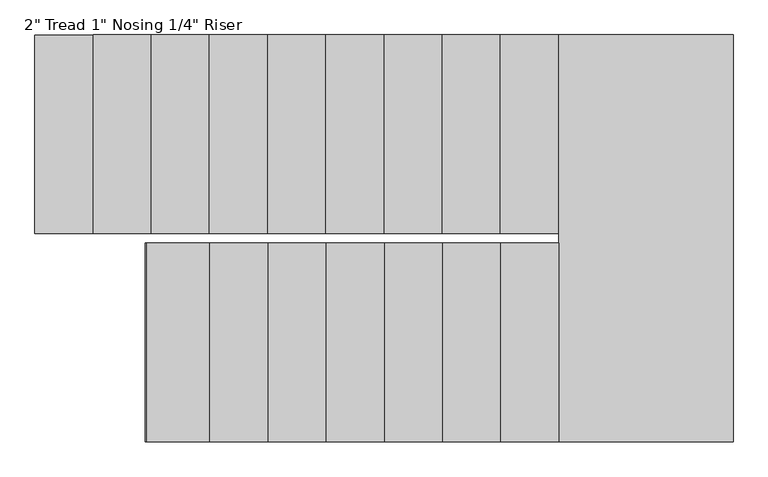
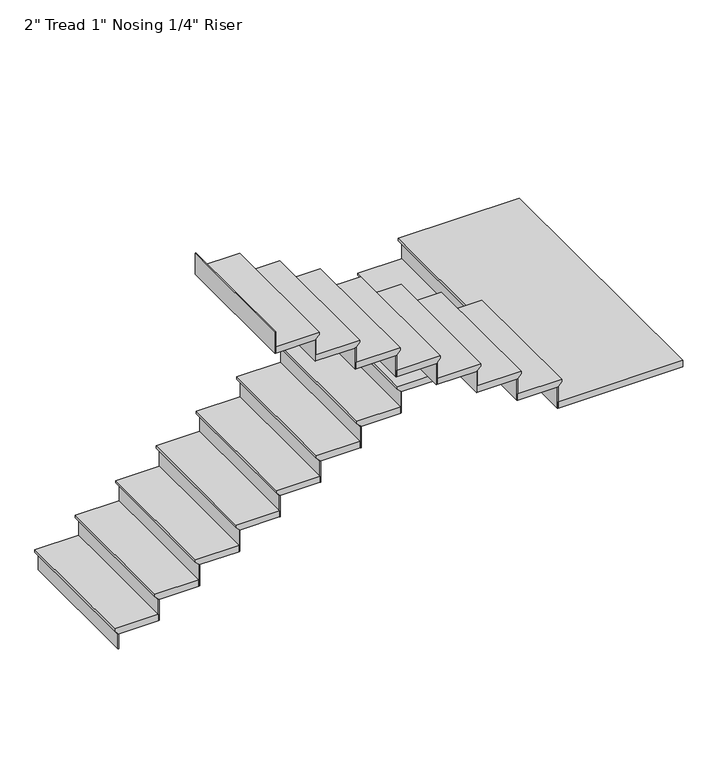
"""IFC4 building model written with IfcOpenShell, lengths in millimetres: stair flight geometry."""

from ifc_helpers import new_model, si_unit, origin, place, context, project, spatial, faceted_brep, source, transform, mapped, element, save


def stair_flight_e0aa27d8(model_context):
    return source(origin(), model_context, "Body", "Brep", [
        faceted_brep([(1775.9671209, 2655.5223211, 455.0833333), (1775.9671209, 2655.5223211, 474.1333333), (1775.9671209, 3696.9223211, 474.1333333), (1775.9671209, 3696.9223211, 455.0833333), (1801.3671209, 2655.5223211, 429.6833333), (1801.3671209, 3696.9223211, 429.6833333), (2106.1671209, 2655.5223211, 474.1333333), (2106.1671209, 3696.9223211, 474.1333333), (1801.3671209, 3696.9223211, 423.3333333), (2106.1671209, 3696.9223211, 423.3333333), (2106.1671209, 2655.5223211, 423.3333333), (1801.3671209, 2655.5223211, 423.3333333)], [[[0, 1, 2, 3]], [[4, 0, 3, 5]], [[2, 1, 6, 7]], [[8, 9, 10, 11]], [[2, 7, 9, 8, 5, 3]], [[8, 11, 4, 5]], [[6, 1, 0, 4, 11, 10]], [[7, 6, 10, 9]]]),
        faceted_brep([(1801.3671209, 2655.5223211, 423.3333333), (1801.3671209, 2655.5223211, 304.8), (1807.7171209, 2655.5223211, 304.8), (1807.7171209, 2655.5223211, 423.3333333), (1801.3671209, 3696.9223211, 423.3333333), (1807.7171209, 3696.9223211, 423.3333333), (1807.7171209, 3696.9223211, 304.8), (1801.3671209, 3696.9223211, 304.8)], [[[0, 1, 2, 3]], [[4, 5, 6, 7]], [[1, 0, 4, 7]], [[2, 1, 7, 6]], [[3, 2, 6, 5]], [[0, 3, 5, 4]]]),
        faceted_brep([(2106.1671209, 2655.5223211, 592.6666667), (2106.1671209, 2655.5223211, 423.3333333), (2112.5171209, 2655.5223211, 423.3333333), (2112.5171209, 2655.5223211, 592.6666667), (2106.1671209, 3696.9223211, 592.6666667), (2112.5171209, 3696.9223211, 592.6666667), (2112.5171209, 3696.9223211, 423.3333333), (2106.1671209, 3696.9223211, 423.3333333)], [[[0, 1, 2, 3]], [[4, 5, 6, 7]], [[1, 0, 4, 7]], [[2, 1, 7, 6]], [[3, 2, 6, 5]], [[0, 3, 5, 4]]]),
        faceted_brep([(2080.7671209, 3696.9223211, 643.4666667), (2080.7671209, 2655.5223211, 643.4666667), (2410.9671209, 2655.5223211, 643.4666667), (2410.9671209, 3696.9223211, 643.4666667), (2106.1671209, 3696.9223211, 592.6666667), (2410.9671209, 3696.9223211, 592.6666667), (2410.9671209, 2655.5223211, 592.6666667), (2106.1671209, 2655.5223211, 592.6666667), (2106.1671209, 3696.9223211, 599.0166667), (2080.7671209, 3696.9223211, 624.4166667), (2106.1671209, 2655.5223211, 599.0166667), (2080.7671209, 2655.5223211, 624.4166667)], [[[0, 1, 2, 3]], [[4, 5, 6, 7]], [[0, 3, 5, 4, 8, 9]], [[4, 7, 10, 8]], [[2, 1, 11, 10, 7, 6]], [[3, 2, 6, 5]], [[11, 1, 0, 9]], [[10, 11, 9, 8]]]),
        faceted_brep([(2410.9671209, 2655.5223211, 762.0), (2410.9671209, 2655.5223211, 592.6666667), (2417.3171209, 2655.5223211, 592.6666667), (2417.3171209, 2655.5223211, 762.0), (2410.9671209, 3696.9223211, 762.0), (2417.3171209, 3696.9223211, 762.0), (2417.3171209, 3696.9223211, 592.6666667), (2410.9671209, 3696.9223211, 592.6666667)], [[[0, 1, 2, 3]], [[4, 5, 6, 7]], [[1, 0, 4, 7]], [[2, 1, 7, 6]], [[3, 2, 6, 5]], [[0, 3, 5, 4]]]),
        faceted_brep([(2385.5671209, 3696.9223211, 812.8), (2385.5671209, 2655.5223211, 812.8), (2715.7671209, 2655.5223211, 812.8), (2715.7671209, 3696.9223211, 812.8), (2410.9671209, 3696.9223211, 762.0), (2715.7671209, 3696.9223211, 762.0), (2715.7671209, 2655.5223211, 762.0), (2410.9671209, 2655.5223211, 762.0), (2410.9671209, 3696.9223211, 768.35), (2385.5671209, 3696.9223211, 793.75), (2410.9671209, 2655.5223211, 768.35), (2385.5671209, 2655.5223211, 793.75)], [[[0, 1, 2, 3]], [[4, 5, 6, 7]], [[0, 3, 5, 4, 8, 9]], [[4, 7, 10, 8]], [[2, 1, 11, 10, 7, 6]], [[3, 2, 6, 5]], [[11, 1, 0, 9]], [[10, 11, 9, 8]]]),
        faceted_brep([(2715.7671209, 2655.5223211, 931.3333333), (2715.7671209, 2655.5223211, 762.0), (2722.1171209, 2655.5223211, 762.0), (2722.1171209, 2655.5223211, 931.3333333), (2715.7671209, 3696.9223211, 931.3333333), (2722.1171209, 3696.9223211, 931.3333333), (2722.1171209, 3696.9223211, 762.0), (2715.7671209, 3696.9223211, 762.0)], [[[0, 1, 2, 3]], [[4, 5, 6, 7]], [[1, 0, 4, 7]], [[2, 1, 7, 6]], [[3, 2, 6, 5]], [[0, 3, 5, 4]]]),
        faceted_brep([(2690.3671209, 3696.9223211, 982.1333333), (2690.3671209, 2655.5223211, 982.1333333), (3020.5671209, 2655.5223211, 982.1333333), (3020.5671209, 3696.9223211, 982.1333333), (2715.7671209, 3696.9223211, 931.3333333), (3020.5671209, 3696.9223211, 931.3333333), (3020.5671209, 2655.5223211, 931.3333333), (2715.7671209, 2655.5223211, 931.3333333), (2715.7671209, 3696.9223211, 937.6833333), (2690.3671209, 3696.9223211, 963.0833333), (2715.7671209, 2655.5223211, 937.6833333), (2690.3671209, 2655.5223211, 963.0833333)], [[[0, 1, 2, 3]], [[4, 5, 6, 7]], [[0, 3, 5, 4, 8, 9]], [[4, 7, 10, 8]], [[2, 1, 11, 10, 7, 6]], [[3, 2, 6, 5]], [[11, 1, 0, 9]], [[10, 11, 9, 8]]]),
        faceted_brep([(3020.5671209, 2655.5223211, 1100.6666667), (3020.5671209, 2655.5223211, 931.3333333), (3026.9171209, 2655.5223211, 931.3333333), (3026.9171209, 2655.5223211, 1100.6666667), (3020.5671209, 3696.9223211, 1100.6666667), (3026.9171209, 3696.9223211, 1100.6666667), (3026.9171209, 3696.9223211, 931.3333333), (3020.5671209, 3696.9223211, 931.3333333)], [[[0, 1, 2, 3]], [[4, 5, 6, 7]], [[1, 0, 4, 7]], [[2, 1, 7, 6]], [[3, 2, 6, 5]], [[0, 3, 5, 4]]]),
        faceted_brep([(2995.1671209, 3696.9223211, 1151.4666667), (2995.1671209, 2655.5223211, 1151.4666667), (3325.3671209, 2655.5223211, 1151.4666667), (3325.3671209, 3696.9223211, 1151.4666667), (3020.5671209, 3696.9223211, 1100.6666667), (3325.3671209, 3696.9223211, 1100.6666667), (3325.3671209, 2655.5223211, 1100.6666667), (3020.5671209, 2655.5223211, 1100.6666667), (3020.5671209, 3696.9223211, 1107.0166667), (2995.1671209, 3696.9223211, 1132.4166667), (3020.5671209, 2655.5223211, 1107.0166667), (2995.1671209, 2655.5223211, 1132.4166667)], [[[0, 1, 2, 3]], [[4, 5, 6, 7]], [[0, 3, 5, 4, 8, 9]], [[4, 7, 10, 8]], [[2, 1, 11, 10, 7, 6]], [[3, 2, 6, 5]], [[11, 1, 0, 9]], [[10, 11, 9, 8]]]),
        faceted_brep([(3325.3671209, 2655.5223211, 1270.0), (3325.3671209, 2655.5223211, 1100.6666667), (3331.7171209, 2655.5223211, 1100.6666667), (3331.7171209, 2655.5223211, 1270.0), (3325.3671209, 3696.9223211, 1270.0), (3331.7171209, 3696.9223211, 1270.0), (3331.7171209, 3696.9223211, 1100.6666667), (3325.3671209, 3696.9223211, 1100.6666667)], [[[0, 1, 2, 3]], [[4, 5, 6, 7]], [[1, 0, 4, 7]], [[2, 1, 7, 6]], [[3, 2, 6, 5]], [[0, 3, 5, 4]]]),
        faceted_brep([(3299.9671209, 3696.9223211, 1320.8), (3299.9671209, 2655.5223211, 1320.8), (3630.1671209, 2655.5223211, 1320.8), (3630.1671209, 3696.9223211, 1320.8), (3325.3671209, 3696.9223211, 1270.0), (3630.1671209, 3696.9223211, 1270.0), (3630.1671209, 2655.5223211, 1270.0), (3325.3671209, 2655.5223211, 1270.0), (3325.3671209, 3696.9223211, 1276.35), (3299.9671209, 3696.9223211, 1301.75), (3325.3671209, 2655.5223211, 1276.35), (3299.9671209, 2655.5223211, 1301.75)], [[[0, 1, 2, 3]], [[4, 5, 6, 7]], [[0, 3, 5, 4, 8, 9]], [[4, 7, 10, 8]], [[2, 1, 11, 10, 7, 6]], [[3, 2, 6, 5]], [[11, 1, 0, 9]], [[10, 11, 9, 8]]]),
        faceted_brep([(3630.1671209, 2655.5223211, 1439.3333333), (3630.1671209, 2655.5223211, 1270.0), (3636.5171209, 2655.5223211, 1270.0), (3636.5171209, 2655.5223211, 1439.3333333), (3630.1671209, 3696.9223211, 1439.3333333), (3636.5171209, 3696.9223211, 1439.3333333), (3636.5171209, 3696.9223211, 1270.0), (3630.1671209, 3696.9223211, 1270.0)], [[[0, 1, 2, 3]], [[4, 5, 6, 7]], [[1, 0, 4, 7]], [[2, 1, 7, 6]], [[3, 2, 6, 5]], [[0, 3, 5, 4]]]),
        faceted_brep([(3604.7671209, 3696.9223211, 1490.1333333), (3604.7671209, 2655.5223211, 1490.1333333), (3934.9671209, 2655.5223211, 1490.1333333), (3934.9671209, 3696.9223211, 1490.1333333), (3630.1671209, 3696.9223211, 1439.3333333), (3934.9671209, 3696.9223211, 1439.3333333), (3934.9671209, 2655.5223211, 1439.3333333), (3630.1671209, 2655.5223211, 1439.3333333), (3630.1671209, 3696.9223211, 1445.6833333), (3604.7671209, 3696.9223211, 1471.0833333), (3630.1671209, 2655.5223211, 1445.6833333), (3604.7671209, 2655.5223211, 1471.0833333)], [[[0, 1, 2, 3]], [[4, 5, 6, 7]], [[0, 3, 5, 4, 8, 9]], [[4, 7, 10, 8]], [[2, 1, 11, 10, 7, 6]], [[3, 2, 6, 5]], [[11, 1, 0, 9]], [[10, 11, 9, 8]]]),
        faceted_brep([(3934.9671209, 2655.5223211, 1608.6666667), (3934.9671209, 2655.5223211, 1439.3333333), (3941.3171209, 2655.5223211, 1439.3333333), (3941.3171209, 2655.5223211, 1608.6666667), (3934.9671209, 3696.9223211, 1608.6666667), (3941.3171209, 3696.9223211, 1608.6666667), (3941.3171209, 3696.9223211, 1439.3333333), (3934.9671209, 3696.9223211, 1439.3333333)], [[[0, 1, 2, 3]], [[4, 5, 6, 7]], [[1, 0, 4, 7]], [[2, 1, 7, 6]], [[3, 2, 6, 5]], [[0, 3, 5, 4]]]),
        faceted_brep([(3909.5671209, 3696.9223211, 1659.4666667), (3909.5671209, 2655.5223211, 1659.4666667), (4239.7671209, 2655.5223211, 1659.4666667), (4239.7671209, 3696.9223211, 1659.4666667), (3934.9671209, 3696.9223211, 1608.6666667), (4239.7671209, 3696.9223211, 1608.6666667), (4239.7671209, 2655.5223211, 1608.6666667), (3934.9671209, 2655.5223211, 1608.6666667), (3934.9671209, 3696.9223211, 1615.0166667), (3909.5671209, 3696.9223211, 1640.4166667), (3934.9671209, 2655.5223211, 1615.0166667), (3909.5671209, 2655.5223211, 1640.4166667)], [[[0, 1, 2, 3]], [[4, 5, 6, 7]], [[0, 3, 5, 4, 8, 9]], [[4, 7, 10, 8]], [[2, 1, 11, 10, 7, 6]], [[3, 2, 6, 5]], [[11, 1, 0, 9]], [[10, 11, 9, 8]]]),
        faceted_brep([(4239.7671209, 2655.5223211, 1778.0), (4239.7671209, 2655.5223211, 1608.6666667), (4246.1171209, 2655.5223211, 1608.6666667), (4246.1171209, 2655.5223211, 1778.0), (4239.7671209, 3696.9223211, 1778.0), (4246.1171209, 3696.9223211, 1778.0), (4246.1171209, 3696.9223211, 1608.6666667), (4239.7671209, 3696.9223211, 1608.6666667)], [[[0, 1, 2, 3]], [[4, 5, 6, 7]], [[1, 0, 4, 7]], [[2, 1, 7, 6]], [[3, 2, 6, 5]], [[0, 3, 5, 4]]]),
        faceted_brep([(4214.3671209, 3696.9223211, 1828.8), (4214.3671209, 2655.5223211, 1828.8), (4544.5671209, 2655.5223211, 1828.8), (4544.5671209, 3696.9223211, 1828.8), (4239.7671209, 3696.9223211, 1778.0), (4544.5671209, 3696.9223211, 1778.0), (4544.5671209, 2655.5223211, 1778.0), (4239.7671209, 2655.5223211, 1778.0), (4239.7671209, 3696.9223211, 1784.35), (4214.3671209, 3696.9223211, 1809.75), (4239.7671209, 2655.5223211, 1784.35), (4214.3671209, 2655.5223211, 1809.75)], [[[0, 1, 2, 3]], [[4, 5, 6, 7]], [[0, 3, 5, 4, 8, 9]], [[4, 7, 10, 8]], [[2, 1, 11, 10, 7, 6]], [[3, 2, 6, 5]], [[11, 1, 0, 9]], [[10, 11, 9, 8]]]),
        faceted_brep([(4544.5671209, 2655.5223211, 1947.3333333), (4544.5671209, 2655.5223211, 1778.0), (4550.9171209, 2655.5223211, 1778.0), (4550.9171209, 2655.5223211, 1947.3333333), (4544.5671209, 3696.9223211, 1947.3333333), (4550.9171209, 3696.9223211, 1947.3333333), (4550.9171209, 3696.9223211, 1778.0), (4544.5671209, 3696.9223211, 1778.0)], [[[0, 1, 2, 3]], [[4, 5, 6, 7]], [[1, 0, 4, 7]], [[2, 1, 7, 6]], [[3, 2, 6, 5]], [[0, 3, 5, 4]]]),
        faceted_brep([(4493.7671209, 1563.3223211, 1998.1333333), (5433.5671209, 1563.3223211, 1998.1333333), (5433.5671209, 3696.9223211, 1998.1333333), (4519.1671209, 3696.9223211, 1998.1333333), (4519.1671209, 2604.7223211, 1998.1333333), (4493.7671209, 2604.7223211, 1998.1333333), (5433.5671209, 1563.3223211, 1947.3333333), (4493.7671209, 1563.3223211, 1947.3333333), (4493.7671209, 2604.7223211, 1947.3333333), (4519.1671209, 2604.7223211, 1947.3333333), (4519.1671209, 2655.5223211, 1947.3333333), (4544.5671209, 2655.5223211, 1947.3333333), (4544.5671209, 3696.9223211, 1947.3333333), (5433.5671209, 3696.9223211, 1947.3333333), (4544.5671209, 3696.9223211, 1953.6833333), (4519.1671209, 3696.9223211, 1979.0833333), (4544.5671209, 2655.5223211, 1953.6833333), (4519.1671209, 2655.5223211, 1979.0833333)], [[[0, 1, 2, 3, 4, 5]], [[6, 7, 8, 9, 10, 11, 12, 13]], [[1, 0, 7, 6]], [[2, 1, 6, 13]], [[3, 2, 13, 12, 14, 15]], [[12, 11, 16, 14]], [[11, 10, 17, 16]], [[4, 3, 15, 17, 10, 9]], [[5, 4, 9, 8]], [[0, 5, 8, 7]], [[15, 14, 16, 17]]]),
        faceted_brep([(4493.7671209, 2604.7223211, 2116.6666667), (4493.7671209, 2604.7223211, 1947.3333333), (4487.4171209, 2604.7223211, 1947.3333333), (4487.4171209, 2604.7223211, 2116.6666667), (4493.7671209, 1563.3223211, 2116.6666667), (4487.4171209, 1563.3223211, 2116.6666667), (4487.4171209, 1563.3223211, 1947.3333333), (4493.7671209, 1563.3223211, 1947.3333333)], [[[0, 1, 2, 3]], [[4, 5, 6, 7]], [[1, 0, 4, 7]], [[2, 1, 7, 6]], [[3, 2, 6, 5]], [[0, 3, 5, 4]]]),
        faceted_brep([(4519.1671209, 1563.3223211, 2167.4666667), (4519.1671209, 2604.7223211, 2167.4666667), (4188.9671209, 2604.7223211, 2167.4666667), (4188.9671209, 1563.3223211, 2167.4666667), (4493.7671209, 1563.3223211, 2116.6666667), (4188.9671209, 1563.3223211, 2116.6666667), (4188.9671209, 2604.7223211, 2116.6666667), (4493.7671209, 2604.7223211, 2116.6666667), (4493.7671209, 1563.3223211, 2123.0166667), (4519.1671209, 1563.3223211, 2148.4166667), (4493.7671209, 2604.7223211, 2123.0166667), (4519.1671209, 2604.7223211, 2148.4166667)], [[[0, 1, 2, 3]], [[4, 5, 6, 7]], [[0, 3, 5, 4, 8, 9]], [[4, 7, 10, 8]], [[2, 1, 11, 10, 7, 6]], [[3, 2, 6, 5]], [[11, 1, 0, 9]], [[10, 11, 9, 8]]]),
        faceted_brep([(4188.9671209, 2604.7223211, 2286.0), (4188.9671209, 2604.7223211, 2116.6666667), (4182.6171209, 2604.7223211, 2116.6666667), (4182.6171209, 2604.7223211, 2286.0), (4188.9671209, 1563.3223211, 2286.0), (4182.6171209, 1563.3223211, 2286.0), (4182.6171209, 1563.3223211, 2116.6666667), (4188.9671209, 1563.3223211, 2116.6666667)], [[[0, 1, 2, 3]], [[4, 5, 6, 7]], [[1, 0, 4, 7]], [[2, 1, 7, 6]], [[3, 2, 6, 5]], [[0, 3, 5, 4]]]),
        faceted_brep([(4214.3671209, 1563.3223211, 2336.8), (4214.3671209, 2604.7223211, 2336.8), (3884.1671209, 2604.7223211, 2336.8), (3884.1671209, 1563.3223211, 2336.8), (4188.9671209, 1563.3223211, 2286.0), (3884.1671209, 1563.3223211, 2286.0), (3884.1671209, 2604.7223211, 2286.0), (4188.9671209, 2604.7223211, 2286.0), (4188.9671209, 1563.3223211, 2292.35), (4214.3671209, 1563.3223211, 2317.75), (4188.9671209, 2604.7223211, 2292.35), (4214.3671209, 2604.7223211, 2317.75)], [[[0, 1, 2, 3]], [[4, 5, 6, 7]], [[0, 3, 5, 4, 8, 9]], [[4, 7, 10, 8]], [[2, 1, 11, 10, 7, 6]], [[3, 2, 6, 5]], [[11, 1, 0, 9]], [[10, 11, 9, 8]]]),
        faceted_brep([(3884.1671209, 2604.7223211, 2455.3333333), (3884.1671209, 2604.7223211, 2286.0), (3877.8171209, 2604.7223211, 2286.0), (3877.8171209, 2604.7223211, 2455.3333333), (3884.1671209, 1563.3223211, 2455.3333333), (3877.8171209, 1563.3223211, 2455.3333333), (3877.8171209, 1563.3223211, 2286.0), (3884.1671209, 1563.3223211, 2286.0)], [[[0, 1, 2, 3]], [[4, 5, 6, 7]], [[1, 0, 4, 7]], [[2, 1, 7, 6]], [[3, 2, 6, 5]], [[0, 3, 5, 4]]]),
        faceted_brep([(3909.5671209, 1563.3223211, 2506.1333333), (3909.5671209, 2604.7223211, 2506.1333333), (3579.3671209, 2604.7223211, 2506.1333333), (3579.3671209, 1563.3223211, 2506.1333333), (3884.1671209, 1563.3223211, 2455.3333333), (3579.3671209, 1563.3223211, 2455.3333333), (3579.3671209, 2604.7223211, 2455.3333333), (3884.1671209, 2604.7223211, 2455.3333333), (3884.1671209, 1563.3223211, 2461.6833333), (3909.5671209, 1563.3223211, 2487.0833333), (3884.1671209, 2604.7223211, 2461.6833333), (3909.5671209, 2604.7223211, 2487.0833333)], [[[0, 1, 2, 3]], [[4, 5, 6, 7]], [[0, 3, 5, 4, 8, 9]], [[4, 7, 10, 8]], [[2, 1, 11, 10, 7, 6]], [[3, 2, 6, 5]], [[11, 1, 0, 9]], [[10, 11, 9, 8]]]),
        faceted_brep([(3579.3671209, 2604.7223211, 2624.6666667), (3579.3671209, 2604.7223211, 2455.3333333), (3573.0171209, 2604.7223211, 2455.3333333), (3573.0171209, 2604.7223211, 2624.6666667), (3579.3671209, 1563.3223211, 2624.6666667), (3573.0171209, 1563.3223211, 2624.6666667), (3573.0171209, 1563.3223211, 2455.3333333), (3579.3671209, 1563.3223211, 2455.3333333)], [[[0, 1, 2, 3]], [[4, 5, 6, 7]], [[1, 0, 4, 7]], [[2, 1, 7, 6]], [[3, 2, 6, 5]], [[0, 3, 5, 4]]]),
        faceted_brep([(3604.7671209, 1563.3223211, 2675.4666667), (3604.7671209, 2604.7223211, 2675.4666667), (3274.5671209, 2604.7223211, 2675.4666667), (3274.5671209, 1563.3223211, 2675.4666667), (3579.3671209, 1563.3223211, 2624.6666667), (3274.5671209, 1563.3223211, 2624.6666667), (3274.5671209, 2604.7223211, 2624.6666667), (3579.3671209, 2604.7223211, 2624.6666667), (3579.3671209, 1563.3223211, 2631.0166667), (3604.7671209, 1563.3223211, 2656.4166667), (3579.3671209, 2604.7223211, 2631.0166667), (3604.7671209, 2604.7223211, 2656.4166667)], [[[0, 1, 2, 3]], [[4, 5, 6, 7]], [[0, 3, 5, 4, 8, 9]], [[4, 7, 10, 8]], [[2, 1, 11, 10, 7, 6]], [[3, 2, 6, 5]], [[11, 1, 0, 9]], [[10, 11, 9, 8]]]),
        faceted_brep([(3274.5671209, 2604.7223211, 2794.0), (3274.5671209, 2604.7223211, 2624.6666667), (3268.2171209, 2604.7223211, 2624.6666667), (3268.2171209, 2604.7223211, 2794.0), (3274.5671209, 1563.3223211, 2794.0), (3268.2171209, 1563.3223211, 2794.0), (3268.2171209, 1563.3223211, 2624.6666667), (3274.5671209, 1563.3223211, 2624.6666667)], [[[0, 1, 2, 3]], [[4, 5, 6, 7]], [[1, 0, 4, 7]], [[2, 1, 7, 6]], [[3, 2, 6, 5]], [[0, 3, 5, 4]]]),
        faceted_brep([(3299.9671209, 1563.3223211, 2844.8), (3299.9671209, 2604.7223211, 2844.8), (2969.7671209, 2604.7223211, 2844.8), (2969.7671209, 1563.3223211, 2844.8), (3274.5671209, 1563.3223211, 2794.0), (2969.7671209, 1563.3223211, 2794.0), (2969.7671209, 2604.7223211, 2794.0), (3274.5671209, 2604.7223211, 2794.0), (3274.5671209, 1563.3223211, 2800.35), (3299.9671209, 1563.3223211, 2825.75), (3274.5671209, 2604.7223211, 2800.35), (3299.9671209, 2604.7223211, 2825.75)], [[[0, 1, 2, 3]], [[4, 5, 6, 7]], [[0, 3, 5, 4, 8, 9]], [[4, 7, 10, 8]], [[2, 1, 11, 10, 7, 6]], [[3, 2, 6, 5]], [[11, 1, 0, 9]], [[10, 11, 9, 8]]]),
        faceted_brep([(2969.7671209, 2604.7223211, 2963.3333333), (2969.7671209, 2604.7223211, 2794.0), (2963.4171209, 2604.7223211, 2794.0), (2963.4171209, 2604.7223211, 2963.3333333), (2969.7671209, 1563.3223211, 2963.3333333), (2963.4171209, 1563.3223211, 2963.3333333), (2963.4171209, 1563.3223211, 2794.0), (2969.7671209, 1563.3223211, 2794.0)], [[[0, 1, 2, 3]], [[4, 5, 6, 7]], [[1, 0, 4, 7]], [[2, 1, 7, 6]], [[3, 2, 6, 5]], [[0, 3, 5, 4]]]),
        faceted_brep([(2995.1671209, 1563.3223211, 3014.1333333), (2995.1671209, 2604.7223211, 3014.1333333), (2664.9671209, 2604.7223211, 3014.1333333), (2664.9671209, 1563.3223211, 3014.1333333), (2969.7671209, 1563.3223211, 2963.3333333), (2664.9671209, 1563.3223211, 2963.3333333), (2664.9671209, 2604.7223211, 2963.3333333), (2969.7671209, 2604.7223211, 2963.3333333), (2969.7671209, 1563.3223211, 2969.6833333), (2995.1671209, 1563.3223211, 2995.0833333), (2969.7671209, 2604.7223211, 2969.6833333), (2995.1671209, 2604.7223211, 2995.0833333)], [[[0, 1, 2, 3]], [[4, 5, 6, 7]], [[0, 3, 5, 4, 8, 9]], [[4, 7, 10, 8]], [[2, 1, 11, 10, 7, 6]], [[3, 2, 6, 5]], [[11, 1, 0, 9]], [[10, 11, 9, 8]]]),
        faceted_brep([(2664.9671209, 2604.7223211, 3132.6666667), (2664.9671209, 2604.7223211, 2963.3333333), (2658.6171209, 2604.7223211, 2963.3333333), (2658.6171209, 2604.7223211, 3132.6666667), (2664.9671209, 1563.3223211, 3132.6666667), (2658.6171209, 1563.3223211, 3132.6666667), (2658.6171209, 1563.3223211, 2963.3333333), (2664.9671209, 1563.3223211, 2963.3333333)], [[[0, 1, 2, 3]], [[4, 5, 6, 7]], [[1, 0, 4, 7]], [[2, 1, 7, 6]], [[3, 2, 6, 5]], [[0, 3, 5, 4]]]),
        faceted_brep([(2360.1671209, 2604.7223211, 3302.0), (2360.1671209, 2604.7223211, 3132.6666667), (2353.8171209, 2604.7223211, 3132.6666667), (2353.8171209, 2604.7223211, 3302.0), (2360.1671209, 1563.3223211, 3302.0), (2353.8171209, 1563.3223211, 3302.0), (2353.8171209, 1563.3223211, 3132.6666667), (2360.1671209, 1563.3223211, 3132.6666667)], [[[0, 1, 2, 3]], [[4, 5, 6, 7]], [[1, 0, 4, 7]], [[2, 1, 7, 6]], [[3, 2, 6, 5]], [[0, 3, 5, 4]]]),
        faceted_brep([(2690.3671209, 1563.3223211, 3183.4666667), (2690.3671209, 2604.7223211, 3183.4666667), (2360.1671209, 2604.7223211, 3183.4666667), (2360.1671209, 1563.3223211, 3183.4666667), (2664.9671209, 1563.3223211, 3132.6666667), (2360.1671209, 1563.3223211, 3132.6666667), (2360.1671209, 2604.7223211, 3132.6666667), (2664.9671209, 2604.7223211, 3132.6666667), (2664.9671209, 1563.3223211, 3139.0166667), (2690.3671209, 1563.3223211, 3164.4166667), (2664.9671209, 2604.7223211, 3139.0166667), (2690.3671209, 2604.7223211, 3164.4166667)], [[[0, 1, 2, 3]], [[4, 5, 6, 7]], [[0, 3, 5, 4, 8, 9]], [[4, 7, 10, 8]], [[2, 1, 11, 10, 7, 6]], [[3, 2, 6, 5]], [[11, 1, 0, 9]], [[10, 11, 9, 8]]]),
    ])


if __name__ == "__main__":
    model = new_model("IFC4")
    model_context = context("Model", 3, world=origin())
    ifc_project = project(units=[si_unit("LENGTHUNIT", "METRE", prefix="MILLI")], contexts=[model_context])
    site = spatial("IfcSite", under=ifc_project)
    building = spatial("IfcBuilding", under=site)
    placement = place(None, origin())
    stair_flight_shape = stair_flight_e0aa27d8(model_context)
    element("IfcStairFlight", 1, ObjectType="2\" Tread 1\" Nosing 1/4\" Riser", at=placement, inside=building, context=model_context, shape_type="MappedRepresentation", body=[
        mapped(stair_flight_shape, transform((0.0, 0.0, 0.0), x_axis=(1.0, 0.0, 0.0), y_axis=(0.0, 1.0, 0.0), z_axis=(0.0, 0.0, 1.0))),
    ])
    save(model, "model.ifc")
